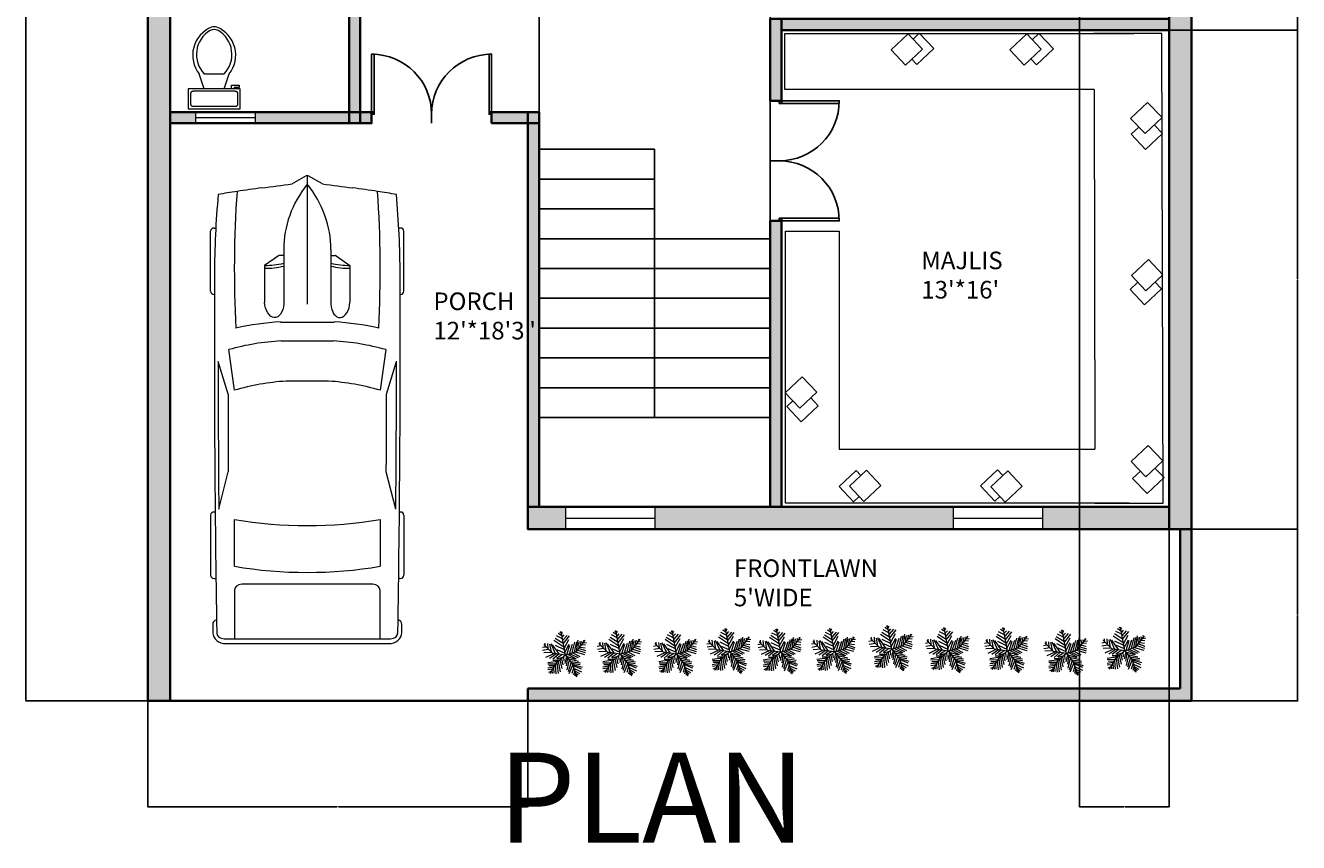
# Model space of a CAD drawing. Units: inches. Extents: x 2119 to 2631, y 2040 to 2935.
# Tile 1 of 3: x 2119 to 2631, y 2040 to 2369. Entities that reach past the tile are written whole.
import ezdxf

# ---------------------------------------------------------------- set-up
doc = ezdxf.new("R2010")
doc.units = ezdxf.units.IN
for name, color, linetype, lineweight in [('A-ANNO-DIMS', 2, 'Continuous', 18), ('A-ANNO-TEXT', 7, 'Continuous', 25), ('A-AREA-IDEN', 7, 'Continuous', 18), ('A-FLOR-FIXT', 9, 'Continuous', 18), ('A-FLOR-STRS', 7, 'Continuous', 25), ('A-WALL-PATT', 252, 'Continuous', 13), ('C-PRKG-VEHI', 8, 'Continuous', 13), ('C-PROP', 7, 'Continuous', 35), ('DOOR', 50, 'Continuous', 25), ('FURNITURE', 220, 'Continuous', 18), ('GRASS', 70, 'Continuous', 13), ('WALL', 180, 'Continuous', 35), ('WINDOW', 130, 'Continuous', 18)]:
    doc.layers.add(name, color=color, linetype=linetype, lineweight=lineweight)
doc.styles.get("Standard").update_dxf_attribs({"font": 'arial.ttf'})
doc.dimstyles.get("Standard").update_dxf_attribs({"dimtxt": 0.18, "dimasz": 0.18, "dimexe": 0.18, "dimexo": 0.0625, "dimgap": 0.09, "dimtad": 0, "dimtih": 1, "dimtoh": 1, "dimdec": 4, "dimzin": 0, "dimdsep": 46, "dimtxsty": 'Standard', "dimcen": 0.09, "dimadec": 0, "dimazin": 0, "dimtfac": 1, "dimtdec": 4, "dimtofl": 0, "dimtmove": 0, "dimatfit": 3, "dimfxl": 1, "dimtolj": 1, "dimtzin": 0, "dimarcsym": 0})

# ---------------------------------------------------------------- blocks, each defined once
blk = doc.blocks.new('*U4')
for p, q in [((9.5, -6), (9.5, -2)), ((-10, -8.5), (-8, -8.5)), ((-10, -9.5), (-10, -8.5)), ((-7, -9.5), (-10, -9.5)), ((-8, -8.5), (-8, -8)), ((-7, -8), (-7, -9.5)), ((-4, -8), (-6, -14)), ((4, -8), (6, -14)), ((4, -14), (-4, -14))]:
    blk.add_line(p, q)
blk.add_lwpolyline([(10.5, -8), (10.5, 0), (-10.5, 0), (-10.5, -8)], close=True)
for points in [[(-9.5, -2), (-9.5, -6)], [(8.5, -1), (-8.5, -1)], [(-8.5, -7), (8.5, -7)]]:
    blk.add_lwpolyline(points)
for centre, radius, start, end in [((-8.62, -1.88), 0.884, 81.8699, 188.1301), ((8.62, -1.88), 0.884, 351.8699, 98.1301), ((-8.62, -6.12), 0.884, 171.8699, 278.1301), ((8.62, -6.12), 0.884, 261.8699, 8.1301), ((3.52, -21.58), 12.17, 141.4691, 247.9714), ((4.2, -21.82), 11.33, 136.3677, 238.9468), ((-3.52, -21.58), 12.17, 292.0284, 38.5307), ((-4.2, -21.82), 11.33, 301.053, 43.6321), ((0, -27.88), 4, 245.7318, 294.2682), ((0, -29), 4, 254.8605, 285.1395)]:
    blk.add_arc(centre, radius, start, end)
blk = doc.blocks.new('*U2')
for p, q in [((0, 0), (0, -6)), ((40, 0), (40, -6))]:
    blk.add_line(p, q)
blk.add_lwpolyline([(0, 0), (0, 40), (1.75, 40), (1.75, 0)], close=True)
blk.add_arc((0, 0), 40, 0, 90)
blk = doc.blocks.new('*U6')
for p, q in [((-3.665, 19.273), (-27.574, 35.527)), ((-5.114, 28.097), (-24.676, 40.636)), ((-7.288, 39.707), (-21.778, 46.673)), ((-8.737, 47.138), (-17.069, 52.711)), ((-10.186, 53.64), (-13.084, 55.962)), ((0, 0), (-10.5, 57)), ((-9.099, 51.782), (-6.563, 55.962)), ((-7.65, 43.423), (-2.578, 49.46)), ((-5.839, 35.992), (4.667, 48.067)), ((-5.114, 27.632), (10.463, 46.673)), ((-2.941, 16.486), (8.652, 37.85)), ((16.259, 5.805), (23.142, 31.348)), ((22.055, 7.198), (27.489, 32.277)), ((27, 9), (48, 36)), ((27.127, 9.056), (31.112, 35.992)), ((35.096, 32.741), (37.27, 22.524)), ((38.719, 34.134), (41.979, 28.561)), ((44.153, 36.456), (45.239, 32.741)), ((-47.498, 19.737), (-55.83, 18.344)), ((-40.615, 13.7), (-55.105, 10.913)), ((-31.5, 4.5), (-52.5, 25.5)), ((-33.37, 6.269), (-52.207, 5.34)), ((-48.585, 21.131), (-49.309, 29.026)), ((-28.299, 3.483), (-47.86, -5.805)), ((-43.513, 28.561), (-42.427, 15.558)), ((-38.442, 26.239), (-34.819, 7.663)), ((-21.416, 3.018), (-38.079, -8.128)), ((-35.544, 28.097), (-24.314, 3.947)), ((0, 0), (-31.5, 4.5)), ((-14.533, 2.09), (-30.834, 25.31)), ((-15.982, 2.09), (-30.11, -9.521)), ((-24.314, 23.917), (-2.941, 13.7)), ((0, 0), (-22.5, -19.5)), ((-6.563, 1.161), (-21.416, -8.128)), ((-20.691, 13.7), (-1.129, 4.876)), ((-1.129, 6.734), (9.014, 26.704)), ((0, 0), (27, 9)), ((0, 0), (18, -22.5)), ((3.942, 1.625), (11.187, 24.381)), ((6.478, 1.625), (26.04, -8.592)), ((10.101, 3.483), (17.708, 26.239)), ((11.187, 3.483), (30.749, -5.805)), ((18.07, 5.805), (35.096, -3.483)), ((24.229, 7.663), (46.688, 1.625)), ((29.662, 12.307), (48.137, 6.269)), ((31.836, 30.883), (32.561, 16.486)), ((33.285, 16.486), (48.862, 10.913)), ((36.183, 19.737), (48.137, 17.88)), ((40.53, 25.775), (48.862, 24.846)), ((43.791, 29.954), (51.036, 30.883)), ((-17.431, -15.094), (-42.789, -18.809)), ((-28.299, -29.026), (-42.789, -31.348)), ((-24.314, -21.596), (-42.427, -22.06)), ((-26.849, -26.24), (-40.253, -25.775)), ((-22.5, -19.5), (-37.5, -45)), ((-15.257, -12.772), (-30.11, -12.772)), ((-29.023, -30.884), (-27.936, -43.887)), ((-25.038, -23.918), (-22.865, -45.281)), ((-20.691, -18.345), (-17.793, -44.352)), ((-6.563, -5.805), (-19.967, -9.985)), ((-17.069, -15.094), (-12.721, -40.172)), ((-13.446, -11.378), (-8.737, -32.741)), ((-9.461, -8.592), (-6.201, -23.453)), ((-4.752, -3.483), (-3.665, -14.629)), ((2.493, -3.019), (-1.491, -20.202)), ((1.769, -2.555), (24.229, -9.521)), ((5.029, -6.27), (2.131, -25.775)), ((9.014, -11.378), (3.58, -35.992)), ((14.085, -16.951), (6.478, -40.172)), ((7.565, -9.056), (32.198, -14.629)), ((18.07, -22.524), (8.289, -45.745)), ((12.274, -15.094), (36.907, -18.809)), ((20.244, -30.419), (15.897, -44.816)), ((16.259, -19.738), (36.183, -22.989)), ((18, -22.5), (27, -52.5)), ((18.433, -22.524), (40.53, -29.026)), ((19.157, -25.311), (38.719, -33.206)), ((-30.834, -34.135), (-42.427, -35.528)), ((-34.457, -39.708), (-40.978, -42.494)), ((-32.646, -36.921), (-31.921, -44.352)), ((22.78, -37.85), (19.519, -48.532)), ((21.331, -32.741), (39.081, -40.636)), ((22.78, -38.314), (34.372, -44.816)), ((24.591, -45.745), (23.142, -50.854)), ((24.591, -43.423), (30.749, -47.603)), ((26.764, -49.925), (28.213, -50.854))]:
    blk.add_line(p, q)
blk = doc.blocks.new('*U8')
for p, q in [((21.1, 37.41), (21.1, 36.83)), ((46.55, 38.89), (22.35, 38.89)), ((47.8, 37.39), (47.8, 37.41)), ((87.99, 31.87), (74.76, 35.92)), ((135.45, 37.07), (135.45, 37.41)), ((136.7, 38.89), (160.9, 38.89)), ((162.15, 37.41), (162.15, 36.77)), ((70.03, 31.54), (86.41, 29.35)), ((134.31, 35.6), (119.29, 31.78)), ((186.47, -33.5), (186.47, 33.5)), ((188.4, -32.76), (188.4, 32.76)), ((138.42, 29.35), (157.25, 29.35)), ((164.52, 26.39), (164.52, -26.39)), ((186.47, 29.35), (167.01, 29.35)), ((32.27, 11.63), (36.13, 17.17)), ((36.13, 17.17), (50.94, 17.17)), ((32.12, 9.51), (32.12, 11.15)), ((58.92, -10.77), (58.92, 10.77)), ((66.55, -10.53), (66.55, 10.53)), ((186.47, -10.53), (186.47, 10.53)), ((3.27, 6.13), (0.1, 0.41)), ((29.77, 9.51), (51.68, 9.51)), ((82.74, 8.5), (82.74, -8.5)), ((0, 0), (51.68, 0)), ((0.1, -0.41), (3.27, -6.13)), ((29.77, -9.51), (51.68, -9.51)), ((32.12, -9.51), (32.12, -11.15)), ((32.27, -11.63), (36.13, -17.17)), ((36.13, -17.17), (50.94, -17.17)), ((86.41, -29.35), (70.03, -31.54)), ((157.25, -29.35), (138.42, -29.35)), ((167.01, -29.35), (186.47, -29.35)), ((87.99, -31.87), (74.76, -35.92)), ((134.31, -35.6), (119.29, -31.78)), ((21.1, -37.41), (21.1, -36.83)), ((46.55, -38.89), (22.35, -38.89)), ((47.8, -37.39), (47.8, -37.41)), ((135.45, -37.07), (135.45, -37.41)), ((136.7, -38.89), (160.9, -38.89)), ((162.15, -37.41), (162.15, -36.77))]:
    blk.add_line(p, q)
for centre, major_axis, ratio, start_param, end_param in [((41.19, -490.86), (0, 528.23), 0.842304, 0.00281, 0.075598), ((22.35, 37.41), (0, -1.48), 0.842304, 3.141593, 4.712389), ((64.48, -10555.62), (0, 10593.03), 0.842304, -0.013397, 0.002797), ((46.55, 37.41), (0, 1.48), 0.842304, -1.570796, 0), ((64.48, -10555.62), (0, -10591.55), 0.842304, 3.133765, 3.140441), ((136.7, 37.41), (0, -1.48), 0.842304, 3.141593, 4.712389), ((160.9, 37.41), (0, 1.48), 0.842304, -1.570796, 0), ((180.63, 35.84), (0, 2.22), 0.842304, -0.013017, 1.249894), ((64.48, -10556.36), (0, 10595.31), 0.842304, -0.013397, -0.013017), ((183.98, 33.5), (0, -2.96), 0.842304, 1.570796, 3.128196), ((183.98, 32.76), (0, -5.25), 0.842304, 1.570796, 3.128196), ((266.03, -27.52), (0, 313.31), 0.842304, 1.367076, 1.39176), ((135.29, 5.39), (0, 81.77), 0.842304, 1.245306, 1.50788), ((95.79, -3666.35), (0, -3698.24), 0.842304, 3.134049, 3.144098), ((259.18, -27.52), (0, -305.3), 0.842304, 4.528606, 4.561838), ((37.47, -593.96), (0, -623.33), 0.842304, 3.096046, 3.200911), ((134.4, 5.39), (0, -89.78), 0.842304, 4.449482, 4.652344), ((149.6, 2.8), (0, -79.58), 0.842304, 4.372215, 4.640744), ((17.08, 0), (0, 147.02), 0.842304, 4.511394, 4.913384), ((35.91, 0), (0, 147.02), 0.842304, 4.511394, 4.913384), ((167.01, 26.39), (0, 2.96), 0.842304, 0, 1.570796), ((-204.49, 52.4), (0, -250.96), 0.842304, 1.385369, 1.434372), ((13.04, 17.01), (0, 27.42), 0.842304, 4.435146, 4.718221), ((14.2, 17.01), (0, 27.42), 0.842304, 4.435146, 4.718221), ((50.79, 13.34), (6.34, -0.36), 0.603834, -1.395552, 1.581315), ((32.75, 11.15), (0, 0.74), 0.842304, 0.879714, 1.570796), ((29.77, -46.66), (0, 56.17), 0.842304, 0, 0.590319), ((0.62, 0), (0, -0.74), 0.842304, 4.131459, 5.293319), ((29.77, 46.66), (0, 56.17), 0.842304, 2.551274, 3.141593), ((-204.49, -52.4), (0, 250.96), 0.842304, -1.434372, -1.385369), ((13.04, -17.01), (0, -27.42), 0.842304, 1.564964, 1.848039), ((14.2, -17.01), (0, -27.42), 0.842304, 1.564964, 1.848039), ((149.6, -2.8), (0, -79.58), 0.842304, -1.499151, -1.230623), ((32.75, -11.15), (0, -0.74), 0.842304, 4.712389, 5.403472), ((134.4, -5.39), (0, -89.78), 0.842304, -1.510751, -1.307889), ((135.29, -5.39), (0, -81.77), 0.842304, -1.50788, -1.245306), ((259.18, 27.52), (0, 305.3), 0.842304, 1.721348, 1.754579), ((266.03, 27.52), (0, 313.31), 0.842304, 1.749832, 1.774517), ((37.47, 593.96), (0, -623.33), 0.842304, -0.059319, 0.045547), ((167.01, -26.39), (0, -2.96), 0.842304, 4.712389, 6.283185), ((41.19, 490.86), (0, -528.23), 0.842304, -0.075598, -0.00281), ((64.48, 10555.62), (0, -10591.55), 0.842304, 0.001152, 0.007828), ((95.79, 3666.35), (0, -3698.24), 0.842304, -0.002505, 0.007544), ((183.98, -33.5), (0, 2.96), 0.842304, 3.15499, 4.712389), ((183.98, -32.76), (0, -5.25), 0.842304, 0.013397, 1.570796), ((22.35, -37.41), (0, 1.48), 0.842304, 1.570796, 3.141593), ((64.48, 10555.62), (0, 10593.03), 0.842304, 3.138796, 3.15499), ((46.55, -37.41), (0, -1.48), 0.842304, 0, 1.570796), ((136.7, -37.41), (0, -1.48), 0.842304, -1.570796, 0), ((160.9, -37.41), (0, 1.48), 0.842304, 3.141593, 4.712389), ((180.63, -35.84), (0, -2.22), 0.842304, -1.249894, 0.013017), ((64.48, 10556.36), (0, 10595.31), 0.842304, 3.15461, 3.15499)]:
    blk.add_ellipse(centre, major_axis=major_axis, ratio=ratio, start_param=start_param, end_param=end_param)
at = {"extrusion": (0, 0, -1)}
blk.add_ellipse((50.79, -13.34), major_axis=(6.34, 0.36), ratio=0.603834, start_param=-1.395552, end_param=1.581315, dxfattribs=at)
blk = doc.blocks.new('*D19')
at = {"layer": 'A-ANNO-DIMS', "color": 0, "lineweight": -2, "transparency": 16777216}
for p, q in [((2168.19, 2877.4), (2119.07, 2877.4)), ((2119.25, 2877.22), (2119.25, 2487.58)), ((2119.25, 2097.58), (2119.25, 2487.22)), ((2168.19, 2097.4), (2119.07, 2097.4))]:
    blk.add_line(p, q, dxfattribs=at)
at = {"layer": 'A-ANNO-DIMS', "color": 0, "lineweight": 100, "transparency": 16777216}
for points in [[(2119.22, 2877.22), (2119.28, 2877.22), (2119.25, 2877.4)], [(2119.22, 2097.58), (2119.28, 2097.58), (2119.25, 2097.4)]]:
    blk.add_solid(points, dxfattribs=at)
at = {"layer": 'Defpoints', "color": 0, "lineweight": 100, "transparency": 16777216}
for p in [(2119.25, 2877.4), (2168.25, 2877.4), (2168.25, 2097.4)]:
    blk.add_point(p, dxfattribs=at)
at = {"layer": 'A-ANNO-DIMS', "color": 0, "transparency": 16777216, "insert": (2119.25, 2487.4), "char_height": 0.18, "attachment_point": 5}
blk.add_mtext('\\A1;780', dxfattribs=at)
blk = doc.blocks.new('*D20')
at = {"layer": 'A-ANNO-DIMS', "color": 0, "lineweight": -2, "transparency": 16777216}
for p, q in [((2168.25, 2097.34), (2168.25, 2054.47)), ((2321.25, 2097.34), (2321.25, 2054.47)), ((2168.43, 2054.65), (2244.47, 2054.65)), ((2321.07, 2054.65), (2245.04, 2054.65))]:
    blk.add_line(p, q, dxfattribs=at)
at = {"layer": 'A-ANNO-DIMS', "color": 0, "lineweight": 100, "transparency": 16777216}
for points in [[(2168.43, 2054.68), (2168.43, 2054.62), (2168.25, 2054.65)], [(2321.07, 2054.68), (2321.07, 2054.62), (2321.25, 2054.65)]]:
    blk.add_solid(points, dxfattribs=at)
at = {"layer": 'Defpoints', "color": 0, "lineweight": 100, "transparency": 16777216}
for p in [(2168.25, 2097.4), (2321.25, 2097.4), (2321.25, 2054.65)]:
    blk.add_point(p, dxfattribs=at)
at = {"layer": 'A-ANNO-DIMS', "color": 0, "transparency": 16777216, "insert": (2244.75, 2054.65), "char_height": 0.18, "attachment_point": 5}
blk.add_mtext('\\A1;153', dxfattribs=at)
blk = doc.blocks.new('*D21')
at = {"layer": 'A-ANNO-DIMS', "color": 0, "lineweight": -2, "transparency": 16777216}
for p, q in [((2325.75, 2175.46), (2325.75, 2934.76)), ((2325.93, 2934.58), (2372.04, 2934.58)), ((2418.57, 2934.58), (2372.47, 2934.58)), ((2418.75, 2175.46), (2418.75, 2934.76))]:
    blk.add_line(p, q, dxfattribs=at)
at = {"layer": 'A-ANNO-DIMS', "color": 0, "lineweight": 100, "transparency": 16777216}
for points in [[(2325.93, 2934.61), (2325.93, 2934.55), (2325.75, 2934.58)], [(2418.57, 2934.61), (2418.57, 2934.55), (2418.75, 2934.58)]]:
    blk.add_solid(points, dxfattribs=at)
at = {"layer": 'Defpoints', "color": 0, "lineweight": 100, "transparency": 16777216}
for p in [(2418.75, 2934.58), (2325.75, 2175.4), (2418.75, 2175.4)]:
    blk.add_point(p, dxfattribs=at)
at = {"layer": 'A-ANNO-DIMS', "color": 0, "transparency": 16777216, "insert": (2372.25, 2934.58), "char_height": 0.18, "attachment_point": 5}
blk.add_mtext('\\A1;93', dxfattribs=at)
blk = doc.blocks.new('*D22')
at = {"layer": 'A-ANNO-DIMS', "color": 0, "lineweight": -2, "transparency": 16777216}
for p, q in [((2588.32, 2166.4), (2631.18, 2166.4)), ((2631, 2166.22), (2631, 2132.08)), ((2631, 2097.58), (2631, 2131.72)), ((2588.32, 2097.4), (2631.18, 2097.4))]:
    blk.add_line(p, q, dxfattribs=at)
at = {"layer": 'A-ANNO-DIMS', "color": 0, "lineweight": 100, "transparency": 16777216}
for points in [[(2630.97, 2166.22), (2631.03, 2166.22), (2631, 2166.4)], [(2630.97, 2097.58), (2631.03, 2097.58), (2631, 2097.4)]]:
    blk.add_solid(points, dxfattribs=at)
at = {"layer": 'Defpoints', "color": 0, "lineweight": 100, "transparency": 16777216}
for p in [(2588.25, 2166.4), (2631, 2166.4), (2588.25, 2097.4)]:
    blk.add_point(p, dxfattribs=at)
at = {"layer": 'A-ANNO-DIMS', "color": 0, "transparency": 16777216, "insert": (2631, 2131.9), "char_height": 0.18, "attachment_point": 5}
blk.add_mtext('\\A1;69', dxfattribs=at)
blk = doc.blocks.new('*D23')
at = {"layer": 'A-ANNO-DIMS', "color": 0, "lineweight": -2, "transparency": 16777216}
for p, q in [((2579.32, 2367.4), (2631.18, 2367.4)), ((2631, 2367.22), (2631, 2267.08)), ((2631, 2166.58), (2631, 2266.72)), ((2588.32, 2166.4), (2631.18, 2166.4))]:
    blk.add_line(p, q, dxfattribs=at)
at = {"layer": 'A-ANNO-DIMS', "color": 0, "lineweight": 100, "transparency": 16777216}
for points in [[(2630.97, 2367.22), (2631.03, 2367.22), (2631, 2367.4)], [(2630.97, 2166.58), (2631.03, 2166.58), (2631, 2166.4)]]:
    blk.add_solid(points, dxfattribs=at)
at = {"layer": 'Defpoints', "color": 0, "lineweight": 100, "transparency": 16777216}
for p in [(2579.25, 2367.4), (2631, 2367.4), (2588.25, 2166.4)]:
    blk.add_point(p, dxfattribs=at)
at = {"layer": 'A-ANNO-DIMS', "color": 0, "transparency": 16777216, "insert": (2631, 2266.9), "char_height": 0.18, "attachment_point": 5}
blk.add_mtext('\\A1;201', dxfattribs=at)
blk = doc.blocks.new('*D24')
at = {"layer": 'A-ANNO-DIMS', "color": 0, "lineweight": -2, "transparency": 16777216}
for p, q in [((2588.32, 2528.16), (2631.18, 2528.16)), ((2631, 2527.98), (2631, 2447.96)), ((2631, 2367.58), (2631, 2447.6)), ((2579.32, 2367.4), (2631.18, 2367.4))]:
    blk.add_line(p, q, dxfattribs=at)
at = {"layer": 'A-ANNO-DIMS', "color": 0, "lineweight": 100, "transparency": 16777216}
for points in [[(2630.97, 2527.98), (2631.03, 2527.98), (2631, 2528.16)], [(2630.97, 2367.58), (2631.03, 2367.58), (2631, 2367.4)]]:
    blk.add_solid(points, dxfattribs=at)
at = {"layer": 'Defpoints', "color": 0, "lineweight": 100, "transparency": 16777216}
for p in [(2588.25, 2528.16), (2631, 2528.16), (2579.25, 2367.4)]:
    blk.add_point(p, dxfattribs=at)
at = {"layer": 'A-ANNO-DIMS', "color": 0, "transparency": 16777216, "insert": (2631, 2447.78), "char_height": 0.18, "attachment_point": 5}
blk.add_mtext('\\A1;160.76', dxfattribs=at)
blk = doc.blocks.new('*D31')
at = {"layer": 'A-ANNO-DIMS', "color": 0, "lineweight": -2, "transparency": 16777216}
for p, q in [((2543.25, 2683.84), (2543.25, 2054.47)), ((2579.25, 2683.84), (2579.25, 2054.47)), ((2543.43, 2054.65), (2561.04, 2054.65)), ((2579.07, 2054.65), (2561.47, 2054.65))]:
    blk.add_line(p, q, dxfattribs=at)
at = {"layer": 'A-ANNO-DIMS', "color": 0, "lineweight": 100, "transparency": 16777216}
for points in [[(2543.43, 2054.68), (2543.43, 2054.62), (2543.25, 2054.65)], [(2579.07, 2054.68), (2579.07, 2054.62), (2579.25, 2054.65)]]:
    blk.add_solid(points, dxfattribs=at)
at = {"layer": 'Defpoints', "color": 0, "lineweight": 100, "transparency": 16777216}
for p in [(2543.25, 2683.9), (2579.25, 2683.9), (2579.25, 2054.65)]:
    blk.add_point(p, dxfattribs=at)
at = {"layer": 'A-ANNO-DIMS', "color": 0, "transparency": 16777216, "insert": (2561.25, 2054.65), "char_height": 0.18, "attachment_point": 5}
blk.add_mtext('\\A1;36', dxfattribs=at)

msp = doc.modelspace()

# ---------------------------------------------------------------- hatches: boundary and pattern name
at = {"layer": 'A-WALL-PATT'}
h = msp.add_hatch(color=256, dxfattribs=at)
h.dxf.hatch_style = 1
h.paths.add_polyline_path([(2177.2549, 2868.3983), (2168.2549, 2868.3983), (2168.2549, 2602.8983), (2177.2549, 2602.8983)])
h.paths.add_polyline_path([(2588.2549, 2877.3983), (2579.2549, 2877.3983), (2579.2549, 2868.6805), (2588.2549, 2868.6805)])
h.paths.add_polyline_path([(2579.2549, 2877.3983), (2168.2549, 2877.3983), (2168.2549, 2868.6805), (2579.2549, 2868.6805)])
h.paths.add_polyline_path([(2588.2549, 2868.6805), (2579.2549, 2868.6805), (2579.2549, 2166.3983), (2588.2549, 2166.3983)])
h = msp.add_hatch(color=256, dxfattribs=at)
h.dxf.hatch_style = 1
h.paths.add_polyline_path([(2177.2549, 2430.3983), (2168.2549, 2430.3983), (2168.2549, 2097.3983), (2177.2549, 2097.3983)])
h.paths.add_polyline_path([(2172.7549, 2602.8983), (2168.2549, 2602.8983), (2168.2549, 2430.3983), (2172.7549, 2430.3983)])
h.paths.add_polyline_path([(2229.7549, 2434.8983), (2177.2549, 2434.8983), (2177.2549, 2430.3983), (2229.7549, 2430.3983)])
h.paths.add_polyline_path([(2342.2549, 2434.8983), (2229.7549, 2434.8983), (2229.7549, 2430.3983), (2342.2549, 2430.3983)])
h.paths.add_polyline_path([(2359.6188, 2434.8983), (2346.7549, 2434.8983), (2346.7549, 2430.3983), (2359.6188, 2430.3983)])
h.paths.add_polyline_path([(2346.7549, 2434.8983), (2342.2549, 2434.8983), (2342.2549, 2430.3983), (2346.7549, 2430.3983)])
h.paths.add_polyline_path([(2346.7549, 2602.8983), (2342.2549, 2602.8983), (2342.2549, 2507.872), (2346.7549, 2507.872)])
h.paths.add_polyline_path([(2346.7549, 2609.1862), (2342.2549, 2609.1862), (2342.2549, 2607.3983), (2346.7549, 2607.3983)])
h.paths.add_polyline_path([(2346.7549, 2607.3983), (2342.2549, 2607.3983), (2229.7549, 2607.3983), (2229.7549, 2602.8983), (2346.7549, 2602.8983)])
h = msp.add_hatch(color=256, dxfattribs=at)
h.dxf.hatch_style = 1
h.paths.add_polyline_path([(2538.7549, 2527.8983), (2423.1333, 2527.8983), (2423.1333, 2523.3983), (2538.7549, 2523.3983)])
h.paths.add_polyline_path([(2234.2549, 2602.8983), (2229.7549, 2602.8983), (2229.7549, 2541.8001), (2234.2549, 2541.8001)])
h.paths.add_polyline_path([(2253.7549, 2392.3266), (2249.2549, 2392.3266), (2249.2549, 2334.3983), (2253.7549, 2334.3983)])
h.paths.add_polyline_path([(2249.2549, 2334.3983), (2211.4668, 2334.3983), (2211.4668, 2329.8983), (2249.2549, 2329.8983)])
h.paths.add_polyline_path([(2258.3247, 2334.3983), (2253.7549, 2334.3983), (2253.7549, 2329.8983), (2258.3247, 2329.8983)])
h.paths.add_polyline_path([(2253.7549, 2334.3983), (2249.2549, 2334.3983), (2249.2549, 2329.8983), (2253.7549, 2329.8983)])
h.paths.add_polyline_path([(2187.4668, 2334.3983), (2177.2549, 2334.3983), (2177.2549, 2329.8983), (2187.4668, 2329.8983)])
h.paths.add_polyline_path([(2253.7549, 2430.3983), (2249.2549, 2430.3983), (2249.2549, 2423.2235), (2253.7549, 2423.2235)])
h.paths.add_polyline_path([(2579.2549, 2371.8983), (2423.2549, 2371.8983), (2423.2549, 2367.3983), (2579.2549, 2367.3983)])
h.paths.add_polyline_path([(2423.2549, 2371.8983), (2418.7549, 2371.8983), (2418.7549, 2338.9216), (2423.2549, 2338.9216)])
h = msp.add_hatch(color=256, dxfattribs=at)
h.dxf.hatch_style = 1
h.paths.add_polyline_path([(2321.2549, 2334.3983), (2306.6627, 2334.3983), (2306.6627, 2329.8983), (2321.2549, 2329.8983)])
h.paths.add_polyline_path([(2325.7549, 2334.3983), (2321.2549, 2334.3983), (2321.2549, 2329.8983), (2325.7549, 2329.8983)])
h.paths.add_polyline_path([(2325.7549, 2329.8983), (2321.2549, 2329.8983), (2321.2549, 2175.3983), (2325.7549, 2175.3983)])
h = msp.add_hatch(color=256, dxfattribs=at)
h.dxf.hatch_style = 1
h.paths.add_polyline_path([(2423.2549, 2290.5836), (2418.7549, 2290.5836), (2418.7549, 2175.3983), (2423.2549, 2175.3983)])
h = msp.add_hatch(color=256, dxfattribs=at)
h.dxf.hatch_style = 1
h.paths.add_polyline_path([(2492.3535, 2175.3983), (2372.3184, 2175.3983), (2372.3184, 2166.3983), (2492.3535, 2166.3983)])
h.paths.add_polyline_path([(2579.2549, 2175.3983), (2528.3535, 2175.3983), (2528.3535, 2166.3983), (2579.2549, 2166.3983)])
h.paths.add_polyline_path([(2336.3184, 2175.3983), (2325.7549, 2175.3983), (2325.7549, 2166.3983), (2336.3184, 2166.3983)])
h.paths.add_polyline_path([(2325.7549, 2175.3983), (2321.2549, 2175.3983), (2321.2549, 2166.3983), (2325.7549, 2166.3983)])
h = msp.add_hatch(color=256, dxfattribs=at)
h.dxf.hatch_style = 1
h.paths.add_polyline_path([(2588.2549, 2166.3983), (2583.7549, 2166.3983), (2583.7549, 2102.3506), (2321.2549, 2102.3506), (2321.2549, 2097.3983), (2588.2549, 2097.3983)])

# ---------------------------------------------------------------- linework, layer by layer
at = {"layer": 'A-FLOR-STRS'}
for p, q in [((2325.7549, 2319.3983), (2372.2549, 2319.3983)), ((2372.2549, 2277.7421), (2372.2549, 2319.3983)), ((2325.7549, 2307.3983), (2372.2549, 2307.3983)), ((2325.7549, 2295.3983), (2372.2549, 2295.3983)), ((2325.7549, 2283.3983), (2418.7549, 2283.3983)), ((2372.2549, 2211.3983), (2372.2549, 2280.7503)), ((2325.7549, 2271.3983), (2418.7549, 2271.3983)), ((2325.7549, 2259.3983), (2418.7549, 2259.3983)), ((2325.7549, 2247.3983), (2418.7549, 2247.3983)), ((2325.7549, 2235.3983), (2418.7549, 2235.3983)), ((2325.7549, 2223.3983), (2418.7549, 2223.3983)), ((2325.7549, 2175.3983), (2325.7549, 2211.3983)), ((2325.7549, 2211.3983), (2418.7549, 2211.3983))]:
    msp.add_line(p, q, dxfattribs=at)
at = {"layer": 'C-PROP'}
msp.add_lwpolyline([(2168.2549, 2097.3983), (2588.2549, 2097.3983), (2588.2549, 2877.3983), (2168.2549, 2877.3983)], close=True, dxfattribs=at)
at = {"layer": 'FURNITURE'}
for points in [[(2549.0677, 2343.4099), (2424.5931, 2343.4099), (2424.5931, 2366.0001), (2565.0965, 2366.0001)], [(2475.6937, 2355.6603), (2477.7186, 2353.5132), (2484.5558, 2359.9611), (2478.7573, 2366.1096), (2476.2367, 2363.7326)], [(2523.6687, 2355.7855), (2525.8725, 2353.4486), (2532.7097, 2359.8965), (2526.9113, 2366.0451), (2524.2383, 2363.5243)], [(2549.4633, 2176.8685), (2576.8696, 2176.8685), (2576.4203, 2366.0001), (2549.014, 2366.0001)], [(2549.0677, 2343.4099), (2549.4115, 2198.7023)], [(2567.0915, 2328.3701), (2563.9792, 2325.435), (2569.7777, 2319.2865), (2576.6149, 2325.7344), (2573.3358, 2329.2115)], [(2424.8484, 2198.7023), (2424.8484, 2286.39), (2446.4553, 2286.39), (2446.4553, 2198.7023)], [(2566.7008, 2265.8632), (2563.5885, 2262.9281), (2569.387, 2256.7795), (2576.2242, 2263.2274), (2573.6478, 2265.9593)], [(2427.8398, 2218.1439), (2425.4277, 2215.8691), (2431.2261, 2209.7205), (2438.0633, 2216.1684), (2435.0606, 2219.3524)], [(2563.1665, 2176.8685), (2424.8484, 2176.8685), (2424.8484, 2198.7023)], [(2446.4553, 2198.7023), (2549.4115, 2198.7023)], [(2455.2074, 2188.0795), (2453.3451, 2190.0543), (2446.5079, 2183.6064), (2452.3063, 2177.4578), (2454.5959, 2179.617)], [(2512.318, 2188.0633), (2510.1795, 2190.3309), (2503.3423, 2183.883), (2509.1408, 2177.7344), (2511.1542, 2179.6332)], [(2567.7155, 2189.8537), (2564.6032, 2186.9186), (2570.4017, 2180.77), (2577.2389, 2187.2179), (2573.5995, 2191.077)]]:
    msp.add_lwpolyline(points, dxfattribs=at)
for points in [[(2474.2119, 2365.8797), (2467.3747, 2359.4318), (2473.1732, 2353.2832), (2480.0104, 2359.7311)], [(2522.0344, 2365.8612), (2515.1972, 2359.4133), (2520.9957, 2353.2647), (2527.8329, 2359.7126)], [(2570.6496, 2338.2951), (2563.8124, 2331.8472), (2569.6109, 2325.6987), (2576.4481, 2332.1466)], [(2570.9616, 2275.043), (2564.1244, 2268.5951), (2569.9229, 2262.4465), (2576.7601, 2268.8944)], [(2431.6743, 2227.7758), (2424.8371, 2221.3279), (2430.6355, 2215.1793), (2437.4727, 2221.6272)], [(2570.9133, 2200.1607), (2564.0761, 2193.7128), (2569.8746, 2187.5642), (2576.7118, 2194.0121)], [(2457.4969, 2190.2387), (2450.6598, 2183.7908), (2456.4582, 2177.6422), (2463.2954, 2184.0901)], [(2514.3314, 2189.9621), (2507.4942, 2183.5142), (2513.2927, 2177.3656), (2520.1299, 2183.8135)]]:
    msp.add_lwpolyline(points, close=True, dxfattribs=at)
at = {"layer": 'WALL'}
for p, q in [((2177.2549, 2430.3983), (2177.2549, 2334.3983)), ((2249.2549, 2334.3983), (2249.2549, 2392.3266)), ((2253.7549, 2329.8983), (2253.7549, 2392.3266)), ((2418.7549, 2371.8983), (2418.7549, 2338.9216)), ((2579.2549, 2367.3983), (2423.2549, 2367.3983)), ((2423.2549, 2367.3983), (2423.2549, 2337.8638)), ((2579.2549, 2175.3983), (2579.2549, 2367.3983)), ((2177.2549, 2334.3983), (2249.2549, 2334.3983)), ((2177.2549, 2334.3983), (2259.3825, 2334.3983)), ((2282.488, 2334.3983), (2282.4995, 2334.3983)), ((2305.6049, 2334.3983), (2325.7549, 2334.3983)), ((2325.7549, 2334.3983), (2325.7549, 2175.3983)), ((2177.2549, 2329.8983), (2253.7549, 2329.8983)), ((2177.2549, 2329.8983), (2258.3247, 2329.8983)), ((2282.4837, 2329.8983), (2282.5037, 2329.8983)), ((2306.6627, 2329.8983), (2321.2549, 2329.8983)), ((2321.2549, 2329.8983), (2321.2549, 2166.3983)), ((2418.7549, 2314.7626), (2418.7549, 2314.7426)), ((2423.2549, 2314.7584), (2423.2549, 2314.7468)), ((2418.7549, 2290.5836), (2418.7549, 2175.3983)), ((2423.2549, 2291.6414), (2423.2549, 2175.3983)), ((2579.2549, 2175.3983), (2321.2549, 2175.3983)), ((2579.2549, 2166.3983), (2321.2549, 2166.3983)), ((2579.2549, 2166.3983), (2588.2549, 2166.3983)), ((2583.7549, 2166.3983), (2583.7549, 2102.3506)), ((2177.2549, 2110.3488), (2177.2549, 2097.3983)), ((2583.7549, 2102.3506), (2321.2549, 2102.3506)), ((2321.2549, 2102.3506), (2321.2549, 2097.3983))]:
    msp.add_line(p, q, dxfattribs=at)
for points in [[(2588.2549, 2877.3983), (2579.2549, 2877.3983), (2579.2549, 2166.3983), (2588.2549, 2166.3983)], [(2168.2549, 2097.3983), (2177.2549, 2097.3983), (2177.2549, 2430.3983), (2168.2549, 2430.3983)], [(2249.2549, 2392.3266), (2253.7549, 2392.3266), (2253.7549, 2329.8983), (2249.2549, 2329.8983)], [(2418.7549, 2371.8983), (2423.2549, 2371.8983), (2423.2549, 2338.9216), (2418.7549, 2338.9216)], [(2579.2549, 2371.8983), (2423.2549, 2371.8983), (2423.2549, 2367.3983), (2579.2549, 2367.3983)], [(2258.3247, 2334.3983), (2177.2549, 2334.3983), (2177.2549, 2329.8983), (2258.3247, 2329.8983)], [(2306.6627, 2329.8983), (2325.7549, 2329.8983), (2325.7549, 2334.3983), (2306.6627, 2334.3983)], [(2321.2549, 2175.3983), (2325.7549, 2175.3983), (2325.7549, 2334.3983), (2321.2549, 2334.3983)], [(2418.7549, 2290.5836), (2423.2549, 2290.5836), (2423.2549, 2175.3983), (2418.7549, 2175.3983)], [(2321.2549, 2175.3983), (2579.2549, 2175.3983), (2579.2549, 2166.3983), (2321.2549, 2166.3983)]]:
    msp.add_lwpolyline(points, close=True, dxfattribs=at)
for points in [[(2579.2549, 2166.3983), (2579.2549, 2528.1615)], [(2177.2549, 2434.8983), (2177.2549, 2106.3983)]]:
    msp.add_lwpolyline(points, dxfattribs=at)
at = {"layer": 'WINDOW'}
for p, q in [((2187.4668, 2334.3983), (2187.4668, 2329.8983)), ((2187.4668, 2332.1483), (2211.4668, 2332.1483)), ((2211.4668, 2334.3983), (2211.4668, 2329.8983)), ((2336.3184, 2175.3983), (2336.3184, 2166.3983)), ((2372.3184, 2175.3983), (2372.3184, 2166.3983)), ((2492.3535, 2175.3983), (2492.3535, 2166.3983)), ((2528.3535, 2175.3983), (2528.3535, 2166.3983)), ((2336.3184, 2170.8983), (2372.3184, 2170.8983)), ((2492.3535, 2170.8983), (2528.3535, 2170.8983))]:
    msp.add_line(p, q, dxfattribs=at)

# ---------------------------------------------------------------- block references
at = {"layer": 'A-FLOR-FIXT', "rotation": 180}
msp.add_blockref('*U4', (2194.9979, 2335.7416), dxfattribs=at)
at = {"layer": 'C-PRKG-VEHI', "rotation": 270}
msp.add_blockref('*U8', (2232.4667, 2308.7877), dxfattribs=at)
at = {"layer": 'DOOR', "yscale": 0.6044752396475273, "zscale": 0.6044752396475273}
for p, xscale in [((2258.3247, 2333.5251), 0.6044752396475273), ((2306.6627, 2333.5251), -0.6044752396475273)]:
    msp.add_blockref('*U2', p, dxfattribs=dict(at, xscale=xscale))
at = {"layer": 'DOOR', "yscale": 0.6044752396475273, "zscale": 0.6044752396475273, "rotation": 270}
for p, xscale in [((2422.3818, 2338.9216), 0.6044752396475273), ((2422.3818, 2290.5836), -0.6044752396475273)]:
    msp.add_blockref('*U2', p, dxfattribs=dict(at, xscale=xscale))
at = {"layer": 'GRASS', "xscale": 0.1657890412075336, "yscale": 0.1657890412075336, "zscale": 0.1657890412075336}
for p in [(2402.52, 2117.0753), (2423.0391, 2116.8973), (2444.6804, 2117.0575), (2467.7644, 2118.1787), (2490.484, 2117.3786), (2514.2331, 2117.3786), (2561.4104, 2117.5389), (2336.3146, 2115.742), (2358.44, 2116.1514), (2381.0391, 2116.1514), (2537.9823, 2116.4165)]:
    msp.add_blockref('*U6', p, dxfattribs=at)

# ---------------------------------------------------------------- texts
at = {"layer": 'A-ANNO-TEXT', "insert": (2309.1592, 2076.4677), "char_height": 36.18244, "attachment_point": 1}
msp.add_mtext_dynamic_manual_height_columns('PLAN', width=2979.256201, gutter_width=180.9122, heights=[0], dxfattribs=at)
at = {"layer": 'A-AREA-IDEN', "char_height": 7.08052, "attachment_point": 1}
for s, insert in [("MAJLIS\\P13'*16'", (2479.5822, 2278.2105)), ('PORCH\\P12\'*18\'3"', (2283.2241, 2261.7461)), ("FRONTLAWN\\P5'WIDE", (2404.1482, 2154.2881))]:
    msp.add_mtext_dynamic_manual_height_columns(s, width=32.794808, gutter_width=35.4026, heights=[0], dxfattribs=dict(at, insert=insert))

# ---------------------------------------------------------------- dimensions: what is measured, and where the dimension line sits
at = {"layer": 'A-ANNO-DIMS'}
for base, p1, p2, picture, middle in [((2418.7549, 2934.5786), (2325.7549, 2175.3983), (2418.7549, 2175.3983), '*D21', (2372.2549, 2934.5786)), ((2579.2549, 2054.6483), (2543.2549, 2683.8983), (2579.2549, 2683.8983), '*D31', (2561.2549, 2054.6483)), ((2321.2549, 2054.6483), (2168.2549, 2097.3983), (2321.2549, 2097.3983), '*D20', (2244.7549, 2054.6483))]:
    dim = msp.add_linear_dim(base=base, p1=p1, p2=p2, dimstyle='Standard', override={"dimdec": 0, "dimlfac": 1, "dimrnd": 0, "dimzin": 0, "dimdsep": 46, "dimlunit": 2}, dxfattribs=at)
    dim.commit()
    dim.dimension.update_dxf_attribs({"geometry": picture, "text_midpoint": middle})
for base, p1, p2, override, picture, middle in [((2119.2479, 2877.3983), (2168.2549, 2097.3983), (2168.2549, 2877.3983), {"dimdec": 0, "dimlfac": 1, "dimrnd": 0, "dimzin": 0, "dimdsep": 46, "dimlunit": 2}, '*D19', (2119.2479, 2487.3983)), ((2631.0049, 2528.1615), (2579.2549, 2367.3983), (2588.2549, 2528.1615), {"dimdec": 2, "dimlfac": 1, "dimrnd": 0, "dimzin": 0, "dimdsep": 46, "dimlunit": 2}, '*D24', (2631.0049, 2447.7799)), ((2631.0049, 2367.3983), (2588.2549, 2166.3983), (2579.2549, 2367.3983), {"dimdec": 0, "dimlfac": 1, "dimrnd": 0, "dimzin": 0, "dimdsep": 46, "dimlunit": 2}, '*D23', (2631.0049, 2266.8983)), ((2631.0049, 2166.3983), (2588.2549, 2097.3983), (2588.2549, 2166.3983), {"dimdec": 0, "dimlfac": 1, "dimrnd": 0, "dimzin": 0, "dimdsep": 46, "dimlunit": 2}, '*D22', (2631.0049, 2131.8983))]:
    dim = msp.add_linear_dim(base=base, p1=p1, p2=p2, angle=90, dimstyle='Standard', override=override, dxfattribs=at)
    dim.commit()
    dim.dimension.update_dxf_attribs({"geometry": picture, "text_midpoint": middle})

doc.saveas('drawing.dxf')
